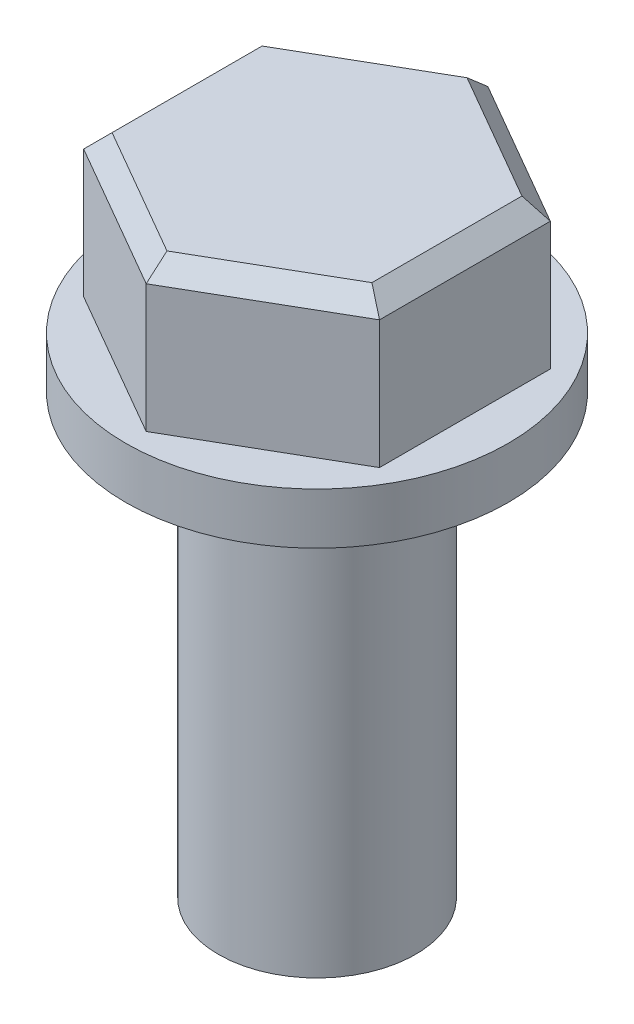
from build123d import *

# Parameters (mm, degrees)
SHANK_SKETCH_12_7_R         = 6.35
SHANK_12_7_DEPTH            = 28.19
FLANGE_SKETCH_24_64_R       = 12.32
FLANGE_24_64_DEPTH          = 3.3
HEX_HEAD_DEPTH              = 9.4
EDGE_CHAMFER_1_16X45_A_SIZE = 1.16
EDGE_CHAMFER_1_16X45_B_SIZE = 1.16
EDGE_CHAMFER_1_16X45_C_SIZE = 1.16


with BuildPart() as part:
    # Shank Sketch Ø12.7 → Shank Ø12.7 (new body)
    with BuildSketch(Plane(origin=(0, 0, 0), x_dir=(1, 0, 0), z_dir=(0, 1, 0))):
        with Locations(Location((0, 0, 0), (0, 0, 90))):
            Circle(SHANK_SKETCH_12_7_R)
    extrude(amount=SHANK_12_7_DEPTH)

    # Flange Sketch Ø24.64 → Flange Ø24.64 (add)
    with BuildSketch(Plane(origin=(0, 28.19, 0), x_dir=(1, 0, 0), z_dir=(0, 1, 0))):
        with Locations(Location((0, 0, 0), (0, 0, 270))):
            Circle(FLANGE_SKETCH_24_64_R)
    extrude(amount=FLANGE_24_64_DEPTH)

    # Hex Head Sketch → Hex Head (add)
    with BuildSketch(Plane(origin=(0, 31.49, 0), x_dir=(1, 0, 0), z_dir=(0, 1, 0))):
        Polygon((0, 11), (-9.526279442, 5.5), (-9.526279442, -5.5), (0, -11), (9.526279442, -5.5), (9.526279442, 5.5), align=None)
    extrude(amount=HEX_HEAD_DEPTH)

    # Edge Chamfer 1.16x45 A
    edge_chamfer_1_16x45_a_edges = [part.edges().sort_by_distance(p)[0] for p in [
        (-9.526279442, 40.89, 0),
        (-4.763139721, 40.89, 8.25),
    ]]
    chamfer(edge_chamfer_1_16x45_a_edges, length=EDGE_CHAMFER_1_16X45_A_SIZE)

    # Edge Chamfer 1.16x45 B
    edge_chamfer_1_16x45_b_edges = [part.edges().sort_by_distance(p)[0] for p in [
        (4.763139721, 40.89, -8.25),
        (9.526279442, 40.89, 0),
        (5.343139721, 40.89, 7.915136844),
    ]]
    chamfer(edge_chamfer_1_16x45_b_edges, length=EDGE_CHAMFER_1_16X45_B_SIZE)

    # Edge Chamfer 1.16x45 C
    edge_chamfer_1_16x45_c_edges = [part.edges().sort_by_distance(p)[0] for p in [
        (-4.763139721, 40.89, -8.25),
    ]]
    chamfer(edge_chamfer_1_16x45_c_edges, length=EDGE_CHAMFER_1_16X45_C_SIZE)


solid = part.part
